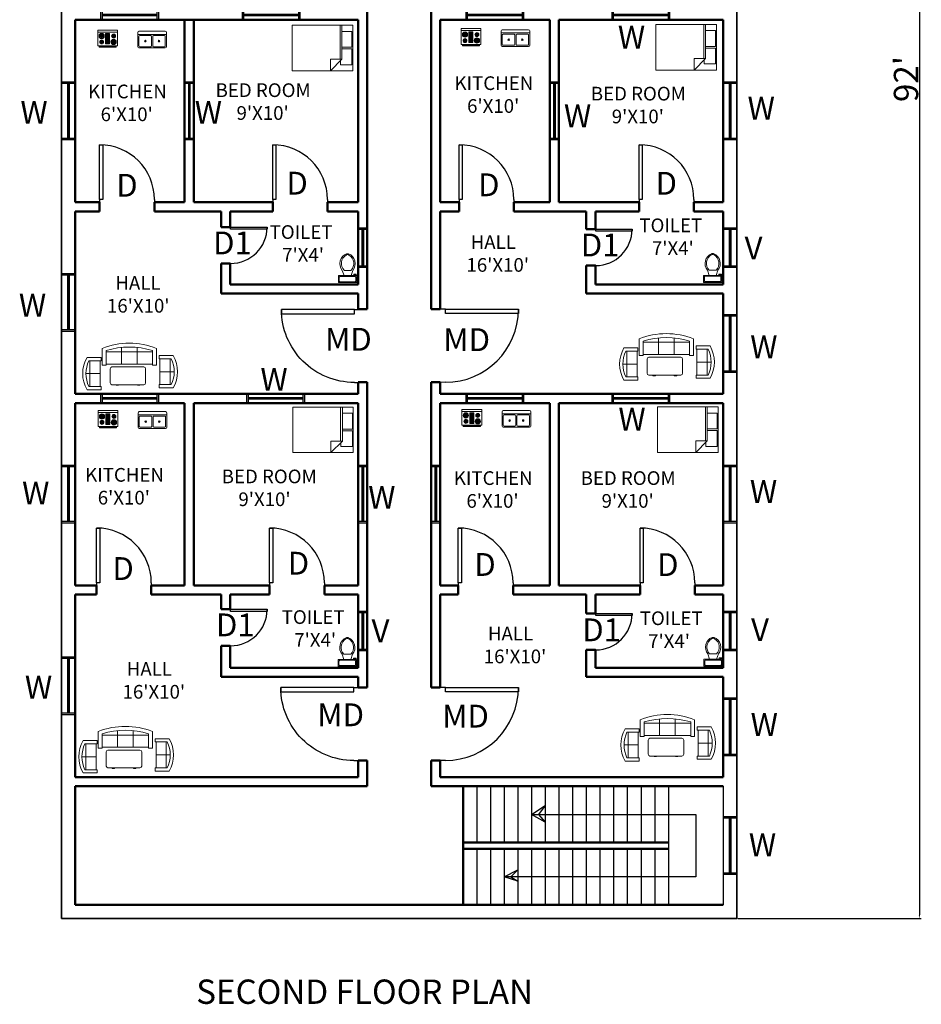
# Model space of a CAD drawing. Units: inches. Extents: x -25308 to -23933, y 10755 to 11996.
# Tile 5 of 6: x -24526 to -23933, y 10755 to 11402. Entities that reach past the tile are written whole.
import ezdxf

# ---------------------------------------------------------------- set-up
doc = ezdxf.new("R2010")
doc.units = ezdxf.units.IN
for name, color, linetype, lineweight in [('A-ANNO-DIMS', 2, 'Continuous', 18), ('A-ANNO-SYMB', 3, 'Continuous', 18), ('A-ANNO-TEXT', 7, 'Continuous', 25), ('A-AREA-IDEN', 7, 'Continuous', 18), ('A-DOOR', 3, 'Continuous', 25), ('A-FLOR-FIXT', 8, 'Continuous', 18), ('A-FLOR-STRS', 2, 'Continuous', 25), ('A-FURN', 8, 'Continuous', 18), ('A-GLAZ', 4, 'Continuous', 25), ('A-WALL', 7, 'Continuous', 50), ('C-PROP', 30, 'Continuous', 35)]:
    doc.layers.add(name, color=color, linetype=linetype, lineweight=lineweight)
doc.styles.get("Standard").update_dxf_attribs({"font": 'arial.ttf'})
doc.dimstyles.new('ISO-25', dxfattribs={"dimtxt": 2.5, "dimasz": 2.5, "dimexe": 1.25, "dimexo": 0.625, "dimtad": 1, "dimdec": 0, "dimlunit": 3, "dimtxsty": 'Standard', "dimcen": 2.5, "dimadec": 0, "dimazin": 0, "dimtfac": 1, "dimtdec": 0, "dimtmove": 0, "dimatfit": 3, "dimfxl": 1, "dimarcsym": 0})

# ---------------------------------------------------------------- blocks, each defined once
blk = doc.blocks.new('*U8')
for p, q in [((0, 0), (0, -100)), ((750, 0), (750, -100))]:
    blk.add_line(p, q)
blk.add_lwpolyline([(0, 0), (0, 750), (43.75, 750), (43.75, 0)], close=True)
blk.add_arc((0, 0), 750, 0, 90)
blk = doc.blocks.new('Range-Oven - 30 in top')
for p, q in [((0, -3), (30, -3)), ((12, -6), (18, -6)), ((13, -20), (13, -6)), ((14, -6), (14, -20)), ((15, -20), (15, -6)), ((16, -6), (16, -20)), ((17, -20), (17, -6)), ((6, -24), (6, -25)), ((8, -25), (8, -24)), ((18, -20), (12, -20)), ((22, -25), (22, -24)), ((24, -24), (24, -25))]:
    blk.add_line(p, q)
for points in [[(0, -24), (0, 0), (30, 0), (30, -24)], [(12, -21), (12, -5), (18, -5), (18, -21)], [(2, -26), (2, -25), (28, -25), (28, -26)]]:
    blk.add_lwpolyline(points, close=True)
for centre, radius in [((6, -9), 4), ((6, -9), 3), ((6, -9), 2), ((6, -9), 1), ((24, -18), 4), ((24, -9), 3), ((24, -9), 2), ((24, -9), 1), ((6, -18), 3), ((6, -18), 2), ((6, -18), 1), ((24, -18), 3), ((24, -18), 2), ((24, -18), 1)]:
    blk.add_circle(centre, radius)
blk = doc.blocks.new('Sink-double - 36 in top')
for p, q in [((-18, -4), (18, -4)), ((-0.75, -18.5), (-0.75, -6.5)), ((0.75, -6.5), (0.75, -18.5))]:
    blk.add_line(p, q)
for points in [[(-16.5, 0), (16.5, 0)], [(-18, -19.5), (-18, -1.5)], [(-16.5, -18.5), (-16.5, -6.5)], [(-15.5, -5.5), (-1.75, -5.5)], [(1.75, -5.5), (15.5, -5.5)], [(16.5, -6.5), (16.5, -18.5)], [(18, -1.5), (18, -19.5)], [(16.5, -21), (-16.5, -21)], [(-1.75, -19.5), (-15.5, -19.5)], [(15.5, -19.5), (1.75, -19.5)]]:
    blk.add_lwpolyline(points)
for centre, radius in [((-8.5, -12.5), 1), ((-8.5, -12.5), 0.5), ((8.5, -12.5), 1), ((8.5, -12.5), 0.5)]:
    blk.add_circle(centre, radius)
for centre, radius, start, end in [((-16.5, -1.5), 1.5, 90, 180), ((16.5, -1.5), 1.5, 0, 90), ((-15.5, -6.5), 1, 90, 180), ((-1.75, -6.5), 1, 0, 90), ((1.75, -6.5), 1, 90, 180), ((15.5, -6.5), 1, 0, 90), ((-16.5, -19.5), 1.5, 180, 270), ((-15.5, -18.5), 1, 180, 270), ((-1.75, -18.5), 1, 270, 0), ((1.75, -18.5), 1, 180, 270), ((15.5, -18.5), 1, 270, 0), ((16.5, -19.5), 1.5, 270, 0)]:
    blk.add_arc(centre, radius, start, end)
blk = doc.blocks.new('Bed - Queen')
for p, q in [((0, -80.00003), (0, 0)), ((0, 0), (59.99999, 0)), ((59.99999, 0), (59.99999, -80.00003)), ((7.99999, -1.2), (28.79998, -1.2)), ((7.99999, -14.4), (7.99999, -1.2)), ((28.79998, -1.2), (28.79998, -14.4)), ((31.19999, -1.2), (51.99999, -1.2)), ((31.19999, -14.4), (31.19999, -1.2)), ((51.99999, -1.2), (51.99999, -16.4)), ((0, -14.4), (44.8, -14.4)), ((44.8, -16.8), (0, -16.8)), ((59.99999, -29.6), (44.8, -14.4)), ((44.8, -14.4), (44.8, -29.6)), ((51.99999, -16.4), (46.79936, -16.4)), ((44.8, -29.6), (59.99999, -29.6)), ((59.99999, -80.00003), (0, -80.00003))]:
    blk.add_line(p, q)
blk = doc.blocks.new('Desk - 30 x 60 in.')
for p, q in [((-26.999995, 0), (26.999995, 0)), ((-29.999995, -27), (-29.999995, -3)), ((29.999995, -3), (29.999995, -27)), ((26.999995, -30), (-26.999995, -30)), ((-20.000005, -30), (-20.000005, -31)), ((-20.000005, -31), (-16.000005, -31)), ((-16.000005, -31), (-16.000005, -30)), ((15.999995, -31), (15.999995, -30)), ((19.999995, -31), (15.999995, -31)), ((19.999995, -30), (19.999995, -31))]:
    blk.add_line(p, q)
for centre, start, end in [((-26.499995, -3.5), 98.1301, 171.8699), ((26.499995, -3.5), 8.130102, 81.8699), ((-26.499995, -26.5), 188.1301, 261.8699), ((26.499995, -26.5), 278.1301, 351.8699)]:
    blk.add_arc(centre, 3.535534, start, end)
blk = doc.blocks.new('Sofa - Roundback 7 ft.')
for p, q in [((-36.000027, -34), (-36.000027, -11.4696)), ((-35.999844, -13.3819), (35.9998, -13.3819)), ((-12.00002, -32.4421), (-12.00003, -6.5971)), ((11.99997, -32.4421), (11.99998, -6.5971)), ((35.99998, -34), (35.99998, -11.4696)), ((-36.000027, -32.4421), (35.99998, -32.4421))]:
    blk.add_line(p, q)
for points in [[(-36.000027, -34), (-42.000027, -34), (-42.000027, -8)], [(41.99998, -8), (41.99998, -34), (35.99998, -34)]]:
    blk.add_lwpolyline(points)
for centre, radius, start, end in [((0, -114.25), 114.25, 68.43141, 111.5686), ((-0.00001, -127.1968), 121.1968, 72.72033, 107.2797)]:
    blk.add_arc(centre, radius, start, end)
blk = doc.blocks.new('Sofa - Roundback Loveseat 5 ft.')
for p, q in [((-24, -33.99998), (-24, -11.46958)), ((-23.9998, -13.38178), (23.99986, -13.38178)), ((0, -32.44198), (0, -5.99998)), ((24.00004, -33.99998), (24.00004, -11.46958)), ((-24, -32.44198), (24.00004, -32.44198))]:
    blk.add_line(p, q)
for points in [[(-24, -33.99998), (-30, -33.99998), (-30, -7.99998)], [(30.00004, -7.99998), (30.00004, -33.99998), (24.00004, -33.99998)]]:
    blk.add_lwpolyline(points)
for centre, radius, start, end in [((0, -60.24998), 60.24998, 60.13715, 119.8628), ((0, -61.38438), 55.38444, 64.32083, 115.6792)]:
    blk.add_arc(centre, radius, start, end)
blk = doc.blocks.new('Toilet - top')
for p, q in [((-10, -8.5), (-8, -8.5)), ((-10, -9.5), (-10, -8.5)), ((-7, -9.5), (-10, -9.5)), ((-8, -8.5), (-8, -8)), ((-7, -8), (-7, -9.5)), ((-4, -8), (-6, -14)), ((4, -8), (6, -14)), ((9.5, -6), (9.5, -2)), ((4, -14), (-4, -14))]:
    blk.add_line(p, q)
blk.add_lwpolyline([(10.5, -8), (10.5, 0), (-10.5, 0), (-10.5, -8)], close=True)
for points in [[(-9.5, -2), (-9.5, -6)], [(8.5, -1), (-8.5, -1)], [(-8.5, -7), (8.5, -7)]]:
    blk.add_lwpolyline(points)
for centre, radius, start, end in [((-8.6, -1.9), 0.884, 81.8699, 188.1301), ((-8.6, -6.1), 0.884, 171.8699, 278.1301), ((8.6, -1.9), 0.884, 351.8699, 98.1301), ((8.6, -6.1), 0.884, 261.8699, 8.1301), ((3.5, -21.6), 12.2, 141.4691, 247.9714), ((4.2, -21.8), 11.3, 136.3677, 238.9468), ((-3.5, -21.6), 12.2, 292.0284, 38.5307), ((-4.2, -21.8), 11.3, 301.053, 43.6321), ((0, -27.9), 4, 245.7318, 294.2682), ((0, -29), 4, 254.8605, 285.1395)]:
    blk.add_arc(centre, radius, start, end)
blk = doc.blocks.new('*D173')
at = {"layer": 'A-ANNO-DIMS', "color": 0, "lineweight": -2, "transparency": 16777216}
for p, q in [((-24053.71, 11915.12), (-23933.08, 11915.12)), ((-23934.33, 11912.62), (-23934.33, 10813.62)), ((-24053.71, 10811.12), (-23933.08, 10811.12))]:
    blk.add_line(p, q, dxfattribs=at)
at = {"layer": 'A-ANNO-DIMS', "color": 0, "transparency": 16777216}
for points in [[(-23934.75, 11912.62), (-23933.91, 11912.62), (-23934.33, 11915.12)], [(-23934.75, 10813.62), (-23933.91, 10813.62), (-23934.33, 10811.12)]]:
    blk.add_solid(points, dxfattribs=at)
at = {"layer": 'Defpoints', "color": 0, "transparency": 16777216}
for p in [(-24054.33, 11915.12), (-24054.33, 10811.12), (-23934.33, 10811.12)]:
    blk.add_point(p, dxfattribs=at)
at = {"layer": 'A-ANNO-DIMS', "color": 0, "transparency": 16777216, "insert": (-23943.13, 11363.12), "char_height": 2.5, "attachment_point": 5, "rotation": 90}
blk.add_mtext("{\\H6.4x;92'}", dxfattribs=at)
blk = doc.blocks.new('WIN-36-9IN')
for p, q in [((0, 9), (0, 0)), ((1, 9), (1, 0)), ((37, 9), (37, 0)), ((38, 9), (38, 0)), ((1, 5), (37, 5)), ((1, 4.5), (37, 4.5)), ((1, 4), (37, 4))]:
    blk.add_line(p, q)
blk = doc.blocks.new('VENT-24')
for p, q in [((0, 26), (9, 26)), ((0, 25), (9, 25)), ((4, 1), (4, 25)), ((4.5, 1), (4.5, 25)), ((5, 1), (5, 25)), ((0, 1), (9, 1)), ((0, 0), (9, 0))]:
    blk.add_line(p, q)
blk = doc.blocks.new('WIN-24-6IN')
for p, q in [((0, 26), (6, 26)), ((0, 25), (6, 25)), ((2.5, 1), (2.5, 25)), ((3, 1), (3, 25)), ((3.5, 1), (3.5, 25)), ((0, 1), (6, 1)), ((0, 0), (6, 0))]:
    blk.add_line(p, q)
blk = doc.blocks.new('WIN-36-6IN')
for p, q in [((0, 6), (0, 0)), ((1, 6), (1, 0)), ((1, 3.5), (37, 3.5)), ((1, 3), (37, 3)), ((1, 2.5), (37, 2.5)), ((37, 6), (37, 0)), ((38, 6), (38, 0))]:
    blk.add_line(p, q)

msp = doc.modelspace()

# ---------------------------------------------------------------- linework, layer by layer
at = {"layer": 'A-FLOR-STRS'}
for p, q in [((-24225.33, 10898.12), (-24225.33, 10861.12)), ((-24216.33, 10898.12), (-24216.33, 10861.12)), ((-24216.33, 10898.12), (-24216.33, 10861.12)), ((-24207.33, 10898.12), (-24207.33, 10861.12)), ((-24198.33, 10898.12), (-24198.33, 10861.12)), ((-24189.33, 10898.12), (-24189.33, 10861.12)), ((-24180.33, 10898.12), (-24180.33, 10861.12)), ((-24171.33, 10898.12), (-24171.33, 10861.12)), ((-24162.33, 10898.12), (-24162.33, 10861.12)), ((-24153.33, 10898.12), (-24153.33, 10861.12)), ((-24144.33, 10898.12), (-24144.33, 10861.12)), ((-24135.33, 10898.12), (-24135.33, 10861.12)), ((-24126.33, 10898.12), (-24126.33, 10861.12)), ((-24117.33, 10898.12), (-24117.33, 10861.12)), ((-24108.33, 10898.12), (-24108.33, 10861.12)), ((-24099.33, 10898.12), (-24099.33, 10820.12)), ((-24063.33, 10898.12), (-24063.33, 10820.12)), ((-24189.33, 10879.62), (-24180.33, 10885.45)), ((-24180.33, 10885.45), (-24184.7, 10879.62)), ((-24189.33, 10879.62), (-24081.37, 10879.62)), ((-24180.33, 10874.63), (-24189.33, 10879.62)), ((-24184.7, 10879.62), (-24180.33, 10874.63)), ((-24081.37, 10879.62), (-24081.37, 10838.62)), ((-24225.33, 10857.12), (-24225.33, 10820.12)), ((-24216.33, 10857.12), (-24216.33, 10820.12)), ((-24216.33, 10857.12), (-24216.33, 10820.12)), ((-24207.33, 10857.12), (-24207.33, 10820.12)), ((-24198.33, 10857.12), (-24198.33, 10820.12)), ((-24189.33, 10857.12), (-24189.33, 10820.12)), ((-24180.33, 10857.12), (-24180.33, 10820.12)), ((-24171.33, 10857.12), (-24171.33, 10820.12)), ((-24162.33, 10857.12), (-24162.33, 10820.12)), ((-24153.33, 10857.12), (-24153.33, 10820.12)), ((-24144.33, 10857.12), (-24144.33, 10820.12)), ((-24135.33, 10857.12), (-24135.33, 10820.12)), ((-24126.33, 10857.12), (-24126.33, 10820.12)), ((-24117.33, 10857.12), (-24117.33, 10820.12)), ((-24108.33, 10857.12), (-24108.33, 10820.12)), ((-24207.33, 10838.62), (-24198.33, 10843.11)), ((-24198.33, 10843.11), (-24202.84, 10838.62)), ((-24081.37, 10838.62), (-24207.33, 10838.62)), ((-24198.33, 10835.83), (-24207.33, 10838.62)), ((-24202.84, 10838.62), (-24198.33, 10835.83))]:
    msp.add_line(p, q, dxfattribs=at)
at = {"layer": 'A-WALL'}
for p, q in [((-24297.33, 11211.71), (-24297.33, 11420.09)), ((-24255.33, 11420.09), (-24255.33, 11211.71)), ((-24489.33, 11402.12), (-24417.33, 11402.12)), ((-24489.33, 11282.12), (-24489.33, 11402.12)), ((-24417.33, 11282.12), (-24417.33, 11402.12)), ((-24417.33, 11402.12), (-24303.33, 11402.12)), ((-24411.33, 11282.12), (-24411.33, 11402.12)), ((-24303.33, 11282.12), (-24303.33, 11402.12)), ((-24249.33, 11402.12), (-24177.33, 11402.12)), ((-24249.33, 11402.12), (-24249.33, 11282.12)), ((-24177.33, 11402.12), (-24177.33, 11282.12)), ((-24171.33, 11402.12), (-24171.33, 11282.12)), ((-24171.33, 11402.12), (-24063.33, 11402.12)), ((-24063.33, 11402.12), (-24063.33, 11282.12)), ((-24489.33, 11282.12), (-24473.21, 11282.12)), ((-24473.21, 11282.12), (-24473.21, 11276.12)), ((-24437.21, 11282.12), (-24437.21, 11276.12)), ((-24437.21, 11282.12), (-24417.33, 11282.12)), ((-24411.33, 11282.12), (-24359.44, 11282.12)), ((-24359.44, 11282.12), (-24359.44, 11276.12)), ((-24323.44, 11282.12), (-24323.44, 11276.12)), ((-24323.44, 11282.12), (-24303.33, 11282.12)), ((-24249.33, 11282.12), (-24236.94, 11282.12)), ((-24236.94, 11282.12), (-24236.94, 11276.12)), ((-24200.94, 11282.12), (-24200.94, 11276.12)), ((-24200.94, 11282.12), (-24177.33, 11282.12)), ((-24171.33, 11282.12), (-24118.59, 11282.12)), ((-24118.59, 11282.12), (-24118.59, 11276.12)), ((-24082.59, 11282.12), (-24082.59, 11276.12)), ((-24082.59, 11282.12), (-24063.33, 11282.12)), ((-24489.33, 11276.12), (-24473.21, 11276.12)), ((-24489.33, 11156.12), (-24489.33, 11276.12)), ((-24437.21, 11276.12), (-24393.33, 11276.12)), ((-24393.33, 11265.82), (-24393.33, 11276.12)), ((-24387.33, 11276.12), (-24359.44, 11276.12)), ((-24387.33, 11265.82), (-24387.33, 11276.12)), ((-24323.44, 11276.12), (-24303.33, 11276.12)), ((-24303.33, 11228.12), (-24303.33, 11276.12)), ((-24249.33, 11276.12), (-24236.94, 11276.12)), ((-24249.33, 11276.12), (-24249.33, 11211.71)), ((-24200.94, 11276.12), (-24153.33, 11276.12)), ((-24153.33, 11276.12), (-24153.33, 11264.44)), ((-24147.33, 11276.12), (-24147.33, 11264.44)), ((-24147.33, 11276.12), (-24118.59, 11276.12)), ((-24082.59, 11276.12), (-24063.33, 11276.12)), ((-24063.33, 11276.12), (-24063.33, 11228.12)), ((-24393.33, 11265.82), (-24387.33, 11265.82)), ((-24153.33, 11264.44), (-24147.33, 11264.44)), ((-24393.33, 11222.12), (-24393.33, 11241.82)), ((-24393.33, 11241.82), (-24387.33, 11241.82)), ((-24387.33, 11228.12), (-24387.33, 11241.82)), ((-24153.33, 11240.44), (-24147.33, 11240.44)), ((-24153.33, 11240.44), (-24153.33, 11222.12)), ((-24147.33, 11240.44), (-24147.33, 11228.12)), ((-24387.33, 11228.12), (-24303.33, 11228.12)), ((-24147.33, 11228.12), (-24063.33, 11228.12)), ((-24393.33, 11222.12), (-24303.33, 11222.12)), ((-24303.33, 11211.71), (-24303.33, 11222.12)), ((-24153.33, 11222.12), (-24063.33, 11222.12)), ((-24063.33, 11222.12), (-24063.33, 11156.12)), ((-24303.33, 11211.71), (-24297.33, 11211.71)), ((-24255.33, 11211.71), (-24249.33, 11211.71)), ((-24303.33, 11156.12), (-24303.33, 11163.71)), ((-24303.33, 11163.71), (-24297.33, 11163.71)), ((-24297.33, 10963.11), (-24297.33, 11163.71)), ((-24255.33, 11163.71), (-24249.33, 11163.71)), ((-24255.33, 11163.71), (-24255.33, 10963.11)), ((-24249.33, 11163.71), (-24249.33, 11156.12)), ((-24489.33, 11156.12), (-24303.33, 11156.12)), ((-24249.33, 11156.12), (-24063.33, 11156.12)), ((-24489.33, 11150.12), (-24417.33, 11150.12)), ((-24489.33, 11030.12), (-24489.33, 11150.12)), ((-24417.33, 11030.12), (-24417.33, 11150.12)), ((-24411.33, 11030.12), (-24411.33, 11150.12)), ((-24411.33, 11150.12), (-24303.33, 11150.12)), ((-24303.33, 11030.12), (-24303.33, 11150.12)), ((-24249.33, 11150.12), (-24177.33, 11150.12)), ((-24249.33, 11150.12), (-24249.33, 11030.12)), ((-24177.33, 11150.12), (-24177.33, 11030.12)), ((-24171.33, 11150.12), (-24171.33, 11030.12)), ((-24171.33, 11150.12), (-24063.33, 11150.12)), ((-24063.33, 11150.12), (-24063.33, 11030.12)), ((-24489.33, 11030.12), (-24475.24, 11030.12)), ((-24489.33, 11024.12), (-24475.24, 11024.12)), ((-24489.33, 10904.12), (-24489.33, 11024.12)), ((-24475.24, 11030.12), (-24475.24, 11024.12)), ((-24439.24, 11030.12), (-24439.24, 11024.12)), ((-24439.24, 11030.12), (-24417.33, 11030.12)), ((-24439.24, 11024.12), (-24393.33, 11024.12)), ((-24411.33, 11030.12), (-24361.46, 11030.12)), ((-24393.33, 11014.48), (-24393.33, 11024.12)), ((-24387.33, 11024.12), (-24361.46, 11024.12)), ((-24387.33, 11014.48), (-24387.33, 11024.12)), ((-24361.46, 11030.12), (-24361.46, 11024.12)), ((-24325.46, 11030.12), (-24325.46, 11024.12)), ((-24325.46, 11030.12), (-24303.33, 11030.12)), ((-24325.46, 11024.12), (-24303.33, 11024.12)), ((-24303.33, 10976.12), (-24303.33, 11024.12)), ((-24249.33, 11030.12), (-24237.45, 11030.12)), ((-24249.33, 11024.12), (-24237.45, 11024.12)), ((-24249.33, 11024.12), (-24249.33, 10963.11)), ((-24237.45, 11030.12), (-24237.45, 11024.12)), ((-24201.45, 11030.12), (-24201.45, 11024.12)), ((-24201.45, 11030.12), (-24177.33, 11030.12)), ((-24201.45, 11024.12), (-24153.33, 11024.12)), ((-24171.33, 11030.12), (-24117.95, 11030.12)), ((-24153.33, 11024.12), (-24153.33, 11011.78)), ((-24147.33, 11024.12), (-24147.33, 11011.78)), ((-24147.33, 11024.12), (-24117.95, 11024.12)), ((-24117.95, 11030.12), (-24117.95, 11024.12)), ((-24081.95, 11030.12), (-24081.95, 11024.12)), ((-24081.95, 11030.12), (-24063.33, 11030.12)), ((-24081.95, 11024.12), (-24063.33, 11024.12)), ((-24063.33, 11024.12), (-24063.33, 10976.12)), ((-24393.33, 11014.48), (-24387.33, 11014.48)), ((-24153.33, 11011.78), (-24147.33, 11011.78)), ((-24393.33, 10970.12), (-24393.33, 10990.48)), ((-24393.33, 10990.48), (-24387.33, 10990.48)), ((-24387.33, 10976.12), (-24387.33, 10990.48)), ((-24153.33, 10987.78), (-24147.33, 10987.78)), ((-24153.33, 10987.78), (-24153.33, 10970.12)), ((-24147.33, 10987.78), (-24147.33, 10976.12)), ((-24387.33, 10976.12), (-24303.33, 10976.12)), ((-24147.33, 10976.12), (-24063.33, 10976.12)), ((-24393.33, 10970.12), (-24303.33, 10970.12)), ((-24303.33, 10963.11), (-24303.33, 10970.12)), ((-24153.33, 10970.12), (-24063.33, 10970.12)), ((-24063.33, 10970.12), (-24063.33, 10904.12)), ((-24303.33, 10963.11), (-24297.33, 10963.11)), ((-24255.33, 10963.11), (-24249.33, 10963.11)), ((-24303.33, 10904.12), (-24303.33, 10915.11)), ((-24303.33, 10915.11), (-24297.33, 10915.11)), ((-24297.33, 10898.12), (-24297.33, 10915.11)), ((-24255.33, 10915.11), (-24249.33, 10915.11)), ((-24255.33, 10915.11), (-24255.33, 10898.12)), ((-24249.33, 10915.11), (-24249.33, 10904.12)), ((-24489.33, 10904.12), (-24303.33, 10904.12)), ((-24249.33, 10904.12), (-24063.33, 10904.12)), ((-24489.33, 10820.12), (-24489.33, 10898.12)), ((-24489.33, 10898.12), (-24297.33, 10898.12)), ((-24255.33, 10898.12), (-24063.33, 10898.12)), ((-24234.33, 10898.12), (-24234.33, 10820.12)), ((-24234.33, 10861.12), (-24099.33, 10861.12)), ((-24234.33, 10857.12), (-24099.33, 10857.12)), ((-24063.33, 10820.12), (-24489.33, 10820.12))]:
    msp.add_line(p, q, dxfattribs=at)
at = {"layer": 'C-PROP'}
for p, q in [((-24498.33, 10811.12), (-24498.33, 11915.12)), ((-24054.33, 11915.12), (-24054.33, 10811.12)), ((-24054.33, 10811.12), (-24498.33, 10811.12))]:
    msp.add_line(p, q, dxfattribs=at)

# ---------------------------------------------------------------- block references
at = {"layer": 'A-DOOR', "xscale": 0.0480000000000013, "yscale": 0.0480000000000013, "zscale": 0.0480000000000013}
for p in [(-24473.21, 11283.92), (-24359.44, 11283.92), (-24236.94, 11283.92), (-24118.59, 11283.92), (-24475.24, 11031.92), (-24361.46, 11031.92), (-24237.45, 11031.92), (-24117.95, 11031.92)]:
    msp.add_blockref('*U8', p, dxfattribs=at)
at = {"layer": 'A-DOOR'}
for p, xscale, yscale, zscale, rotation in [((-24387.13, 11265.82), 0.0320000053173207, 0.0320000053173207, 0.0320000053173207, 270.0087240591115), ((-24147.13, 11264.44), 0.0320000053173207, 0.0320000053173207, 0.0320000053173207, 270.0087240591115), ((-24305.75, 11211.58), -0.0639171163268206, 0.0639171163268206, 0.0639171163268206, 89.99127594088849), ((-24245.93, 11211.71), 0.064000001883637, 0.064000001883637, 0.064000001883637, 270.0087240591115), ((-24387.13, 11014.48), 0.0320000053173207, 0.0320000053173207, 0.0320000053173207, 270.0087240591115), ((-24147.13, 11011.78), 0.0320000053173207, 0.0320000053173207, 0.0320000053173207, 270.0087240591115), ((-24306.17, 10963.01), -0.0639171163268206, 0.0639171163268206, 0.0639171163268206, 89.99127594088849), ((-24245.93, 10963.11), 0.064000001883637, 0.064000001883637, 0.064000001883637, 270.0087240591115)]:
    msp.add_blockref('*U8', p, dxfattribs=dict(at, xscale=xscale, yscale=yscale, zscale=zscale, rotation=rotation))
at = {"layer": 'A-FLOR-FIXT'}
for name, p, xscale, yscale, zscale in [('Range-Oven - 30 in top', (-24474.47, 11395.32), 0.4346134936801813, 0.4346134936801813, 0.4346134936801813), ('Sink-double - 36 in top', (-24438.68, 11394.58), 0.5237879159203632, 0.5237879159203632, 0.5237879159203632), ('Range-Oven - 30 in top', (-24235.63, 11396.26), 0.4346134936801813, 0.4346134936801813, 0.4346134936801813), ('Sink-double - 36 in top', (-24199.85, 11395.51), 0.5237879159203632, 0.5237879159203632, 0.5237879159203632), ('Range-Oven - 30 in top', (-24474.25, 11145.18), 0.4346134936801813, 0.4346134936801813, 0.4346134936801813), ('Sink-double - 36 in top', (-24438.46, 11144.43), 0.5237879159203632, 0.5237879159203632, 0.5237879159203632), ('Range-Oven - 30 in top', (-24235.05, 11145.88), 0.4346134936801813, 0.4346134936801813, 0.4346134936801813), ('Sink-double - 36 in top', (-24199.26, 11145.14), 0.5237879159203632, 0.5237879159203632, 0.5237879159203632)]:
    msp.add_blockref(name, p, dxfattribs=dict(at, xscale=xscale, yscale=yscale, zscale=zscale))
at = {"layer": 'A-FLOR-FIXT', "xscale": 0.5757571651567317, "yscale": 0.5757571651567317, "zscale": 0.5757571651567317, "rotation": 180}
for p in [(-24310.23, 11229.28), (-24070.22, 11229.41), (-24310.4, 10976.94), (-24069.95, 10977.06)]:
    msp.add_blockref('Toilet - top', p, dxfattribs=at)
at = {"layer": 'A-FURN'}
for name, p, xscale, yscale, zscale, rotation in [('Bed - Queen', (-24306.78, 11398.42), 0.4977730924347652, 0.4977730924347652, 0.4977730924347652, 270), ('Bed - Queen', (-24067.67, 11398.91), 0.4977730924347652, 0.4977730924347652, 0.4977730924347652, 270), ('Sofa - Roundback Loveseat 5 ft.', (-24131.37, 11175.74), 0.3543289087725223, 0.3543289087725223, 0.3543289087725223, 89.99999999999999), ('Sofa - Roundback Loveseat 5 ft.', (-24069.1, 11176.99), 0.3543289087725223, 0.3543289087725223, 0.3543289087725223, 270), ('Sofa - Roundback Loveseat 5 ft.', (-24484.33, 11169.43), 0.3543289087725223, 0.3543289087725223, 0.3543289087725223, 89.99999999999999), ('Sofa - Roundback Loveseat 5 ft.', (-24422.06, 11170.68), 0.3543289087725223, 0.3543289087725223, 0.3543289087725223, 270), ('Bed - Queen', (-24306.47, 11147.36), 0.4977730924347652, 0.4977730924347652, 0.4977730924347652, 270), ('Bed - Queen', (-24066.63, 11147.5), 0.4977730924347652, 0.4977730924347652, 0.4977730924347652, 270), ('Sofa - Roundback Loveseat 5 ft.', (-24130.61, 10925.29), 0.3543289087725223, 0.3543289087725223, 0.3543289087725223, 89.99999999999999), ('Sofa - Roundback Loveseat 5 ft.', (-24068.35, 10926.53), 0.3543289087725223, 0.3543289087725223, 0.3543289087725223, 270), ('Sofa - Roundback Loveseat 5 ft.', (-24486.92, 10917.55), 0.3543289087725223, 0.3543289087725223, 0.3543289087725223, 89.99999999999999), ('Sofa - Roundback Loveseat 5 ft.', (-24424.65, 10918.79), 0.3543289087725223, 0.3543289087725223, 0.3543289087725223, 270)]:
    msp.add_blockref(name, p, dxfattribs=dict(at, xscale=xscale, yscale=yscale, zscale=zscale, rotation=rotation))
for name, p, xscale, yscale, zscale in [('Sofa - Roundback 7 ft.', (-24100.72, 11195.74), 0.4248490443916877, 0.4248490443916877, 0.4248490443916877), ('Sofa - Roundback 7 ft.', (-24453.69, 11189.43), 0.4248490443916877, 0.4248490443916877, 0.4248490443916877), ('Desk - 30 x 60 in.', (-24101.67, 11180.15), 0.3893791270499034, 0.3893791270499034, 0.3893791270499034), ('Desk - 30 x 60 in.', (-24454.64, 11173.84), 0.3893791270499034, 0.3893791270499034, 0.3893791270499034), ('Sofa - Roundback 7 ft.', (-24099.97, 10945.28), 0.4248490443916877, 0.4248490443916877, 0.4248490443916877), ('Sofa - Roundback 7 ft.', (-24456.27, 10937.54), 0.4248490443916877, 0.4248490443916877, 0.4248490443916877), ('Desk - 30 x 60 in.', (-24100.92, 10929.69), 0.3893791270499034, 0.3893791270499034, 0.3893791270499034), ('Desk - 30 x 60 in.', (-24457.22, 10921.95), 0.3893791270499034, 0.3893791270499034, 0.3893791270499034)]:
    msp.add_blockref(name, p, dxfattribs=dict(at, xscale=xscale, yscale=yscale, zscale=zscale))
at = {"layer": 'A-GLAZ'}
for name, p, rotation in [('WIN-36-6IN', (-24434.33, 11408.12), 180), ('WIN-36-6IN', (-24341.33, 11408.12), 180), ('WIN-36-6IN', (-24194.33, 11408.12), 180), ('WIN-36-6IN', (-24098.33, 11408.12), 180), ('WIN-36-9IN', (-24498.33, 11361.12), 270.0000000000418), ('WIN-36-6IN', (-24417.33, 11361.12), 270.0000000000161), ('WIN-36-6IN', (-24177.33, 11361.12), 270.0000000000135), ('WIN-36-9IN', (-24063.33, 11361.12), 270.0000000000198), ('WIN-24-6IN', (-24297.33, 11265.12), 180), ('VENT-24', (-24054.33, 11265.12), 180), ('WIN-36-9IN', (-24498.33, 11235.12), 270.0000000000211), ('WIN-36-9IN', (-24063.33, 11208.12), 270.0000000000173), ('WIN-36-6IN', (-24434.33, 11156.12), 180), ('WIN-36-6IN', (-24338.33, 11156.12), 180), ('WIN-36-6IN', (-24194.33, 11156.12), 180), ('WIN-36-6IN', (-24098.33, 11156.12), 180), ('WIN-36-9IN', (-24498.33, 11109.12), 270.0000000000443), ('WIN-36-6IN', (-24303.33, 11109.12), 270.0000000000161), ('WIN-36-6IN', (-24255.33, 11109.12), 270.0000000000135), ('WIN-36-9IN', (-24063.33, 11109.12), 270.0000000000235), ('WIN-24-6IN', (-24297.33, 11013.12), 180), ('VENT-24', (-24054.33, 11013.12), 180), ('WIN-36-9IN', (-24498.33, 10983.12), 270.0000000000173), ('WIN-36-9IN', (-24063.33, 10956.12), 270.0000000000211), ('WIN-36-9IN', (-24063.33, 10878.12), 270.0000000000235)]:
    msp.add_blockref(name, p, dxfattribs=dict(at, rotation=rotation))

# ---------------------------------------------------------------- texts
at = {"layer": 'A-ANNO-SYMB', "char_height": 15, "attachment_point": 1}
for s, insert in [('{W}', (-24132.55, 11398.11)), ('{W}', (-24525.31, 11348.75)), ('{W}', (-24410.68, 11348.75)), ('{W}', (-24047.29, 11351.41)), ('{W}', (-24167.98, 11346.4)), ('{D}', (-24350.43, 11302.13)), ('{D}', (-24462.28, 11300.77)), ('{D}', (-24224.43, 11301.07)), ('{D}', (-24107.78, 11302.08)), ('{D1}', (-24398.62, 11262.86)), ('{D1}', (-24156.94, 11261.52)), ('{V}', (-24049.23, 11259.5)), ('{W}', (-24526.28, 11221.92)), ('{MD}', (-24325.01, 11199.52)), ('{MD}', (-24247.26, 11199.24)), ('{W}', (-24045.57, 11194.59)), ('{W}', (-24367.54, 11173.21)), ('{W}', (-24132.23, 11147.01)), ('{W}', (-24524.18, 11098.44)), ('{W}', (-24296.68, 11095.61)), ('{W}', (-24045.78, 11099.44)), ('{D}', (-24349.56, 11052.28)), ('{D}', (-24226.91, 11051.45)), ('{D}', (-24106.75, 11051.38)), ('{D}', (-24464.8, 11048.77)), ('{D1}', (-24396.72, 11011.75)), ('{V}', (-24294.47, 11007.85)), ('{D1}', (-24155.95, 11008.48)), ('{V}', (-24044.99, 11008.57)), ('{W}', (-24522.33, 10970.76)), ('{MD}', (-24330.09, 10952.63)), ('{MD}', (-24248.03, 10951.74)), ('{W}', (-24045.29, 10946.22)), ('{W}', (-24046.45, 10867.18))]:
    msp.add_mtext_dynamic_manual_height_columns(s, width=853.3083, gutter_width=12.5, heights=[0], dxfattribs=dict(at, insert=insert))
at = {"layer": 'A-ANNO-TEXT', "insert": (-24409.72, 10771.09), "char_height": 16, "attachment_point": 1}
msp.add_mtext_dynamic_manual_height_columns('{SECOND FLOOR PLAN}', width=1113.1425, gutter_width=12.5, heights=[0], dxfattribs=at)
at = {"layer": 'A-AREA-IDEN', "char_height": 9, "attachment_point": 1}
for s, insert in [("{BED ROOM^J     9'X10'}", (-24396.96, 11360.28)), ("{KITCHEN\\P   6'X10'}", (-24239.9, 11364.89)), ("{KITCHEN\\P   6'X10'}", (-24480.81, 11359.43)), ("{ BED ROOM\\P      9'X10'}", (-24153.07, 11358)), ("{     TOILET\\P        7'X4'}", (-24132.16, 11271.42)), ("{  TOILET\\P     7'X4'}", (-24366.96, 11267.02)), ("{ HALL\\P16'X10'}", (-24232.07, 11260.39)), ("{   HALL\\P 16'X10'}", (-24471.12, 11233.56)), ("{KITCHEN\\P   6'X10'}", (-24482.69, 11107.39)), ("{BED ROOM\\P    9'X10'}", (-24392.97, 11106.34)), ("{KITCHEN\\P   6'X10'}", (-24240.34, 11105.25)), ("{BED ROOM\\P     9'X10'}", (-24157.02, 11105.26)), ("{     TOILET\\P        7'X4'}", (-24367.26, 11013.88)), ("{    TOILET\\P      7'X4'}", (-24129.13, 11013.12)), ("{       HALL\\P      16'X10'}", (-24237.21, 11003.01)), ("{        HALL\\P       16'X10'}", (-24477.38, 10979.76))]:
    msp.add_mtext_dynamic_manual_height_columns(s, width=853.3083, gutter_width=12.5, heights=[0], dxfattribs=dict(at, insert=insert))

# ---------------------------------------------------------------- dimensions: what is measured, and where the dimension line sits
at = {"layer": 'A-ANNO-DIMS'}
dim = msp.add_linear_dim(base=(-23934.33, 10811.12), p1=(-24054.33, 11915.12), p2=(-24054.33, 10811.12), angle=90, text='{\\H6.4x;<>}', dimstyle='ISO-25', override={"dimclrd": 0, "dimclre": 0, "dimclrt": 0}, dxfattribs=at)
dim.commit()
dim.dimension.update_dxf_attribs({"geometry": '*D173', "text_midpoint": (-23943.13, 11363.12)})

doc.saveas('drawing.dxf')
